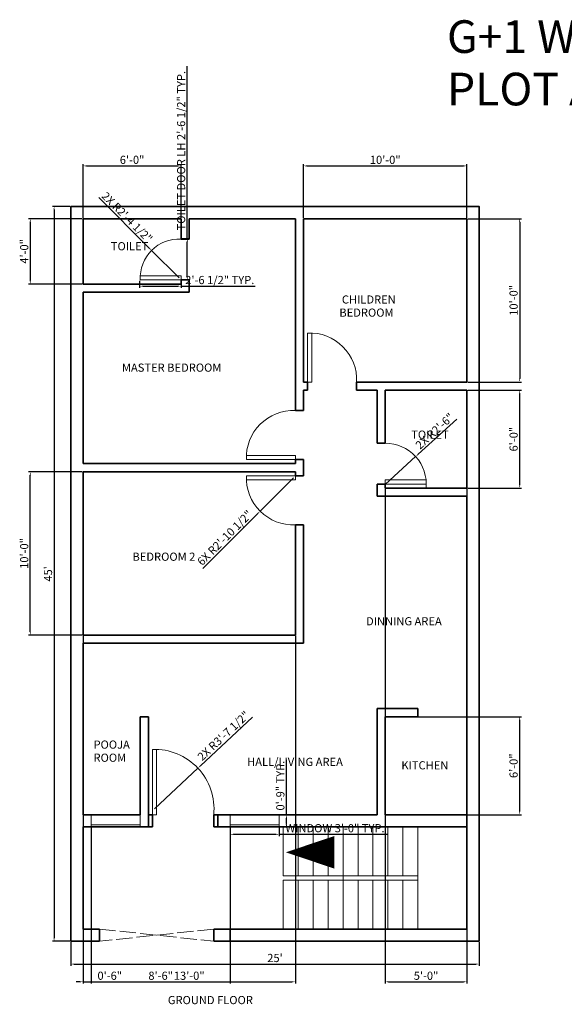
# Model space of a CAD drawing. Units: inches. Extents: x 740 to 2438, y 2555 to 3278.
# Tile 2 of 3: x 1188 to 1588, y 2555 to 3278. Entities that reach past the tile are written whole.
import ezdxf

# ---------------------------------------------------------------- set-up
doc = ezdxf.new("R2010")
doc.units = ezdxf.units.IN
doc.linetypes.add('ACAD_ISO02W100', pattern=[15, 12, -3])
for name, color, linetype, lineweight in [('A-ANNO-DIMS', 2, 'Continuous', 18), ('A-ANNO-TEXT', 7, 'Continuous', 18), ('A-AREA-IDEN', 7, 'Continuous', 18), ('A-DOOR', 3, 'Continuous', 18), ('A-DOOR-SWNG', 3, 'ACAD_ISO02W100', 13), ('A-FLOR-STRS', 7, 'Continuous', 18), ('A-FLOR-STRS-PATH', 2, 'ACAD_ISO02W100', 13), ('A-GLAZ', 4, 'Continuous', 18), ('A-WALL', 7, 'Continuous', 35)]:
    doc.layers.add(name, color=color, linetype=linetype, lineweight=lineweight)
doc.styles.get("Standard").update_dxf_attribs({"font": 'arial.ttf'})
doc.dimstyles.new('ISO-25', dxfattribs={"dimtxt": 6, "dimasz": 2.5, "dimexe": 1.25, "dimexo": 0.625, "dimtad": 1, "dimdec": 1, "dimlunit": 3, "dimtxsty": 'Standard', "dimcen": 2.5, "dimadec": 0, "dimazin": 0, "dimtfac": 1, "dimtdec": 1, "dimtmove": 0, "dimatfit": 3, "dimfxl": 1, "dimarcsym": 0})

# ---------------------------------------------------------------- blocks, each defined once
blk = doc.blocks.new('*D1')
at = {"layer": 'A-ANNO-DIMS', "color": 0, "lineweight": -2, "transparency": 16777216}
for p, q in [((1225.87, 2600.59), (1225.87, 2583.21)), ((1525.87, 2600.59), (1525.87, 2583.21)), ((1228.37, 2584.46), (1523.37, 2584.46))]:
    blk.add_line(p, q, dxfattribs=at)
at = {"layer": 'A-ANNO-DIMS', "color": 0, "transparency": 16777216}
for points in [[(1228.37, 2584.87), (1228.37, 2584.04), (1225.87, 2584.46)], [(1523.37, 2584.87), (1523.37, 2584.04), (1525.87, 2584.46)]]:
    blk.add_solid(points, dxfattribs=at)
at = {"layer": 'Defpoints', "color": 0, "transparency": 16777216}
for p in [(1225.87, 2601.21), (1525.87, 2601.21), (1525.87, 2584.46)]:
    blk.add_point(p, dxfattribs=at)
at = {"layer": 'A-ANNO-DIMS', "color": 0, "transparency": 16777216, "insert": (1375.87, 2588.15), "char_height": 6, "attachment_point": 5}
blk.add_mtext("25'", dxfattribs=at)
blk = doc.blocks.new('*D2')
at = {"layer": 'A-ANNO-DIMS', "color": 0, "lineweight": -2, "transparency": 16777216}
for p, q in [((1225.24, 3141.21), (1212.31, 3141.21)), ((1213.56, 3138.71), (1213.56, 2603.71)), ((1225.24, 2601.21), (1212.31, 2601.21))]:
    blk.add_line(p, q, dxfattribs=at)
at = {"layer": 'A-ANNO-DIMS', "color": 0, "transparency": 16777216}
for points in [[(1213.15, 3138.71), (1213.98, 3138.71), (1213.56, 3141.21)], [(1213.15, 2603.71), (1213.98, 2603.71), (1213.56, 2601.21)]]:
    blk.add_solid(points, dxfattribs=at)
at = {"layer": 'Defpoints', "color": 0, "transparency": 16777216}
for p in [(1225.87, 3141.21), (1213.56, 2601.21), (1225.87, 2601.21)]:
    blk.add_point(p, dxfattribs=at)
at = {"layer": 'A-ANNO-DIMS', "color": 0, "transparency": 16777216, "insert": (1209.89, 2871.21), "char_height": 6, "attachment_point": 5, "rotation": 90}
blk.add_mtext("45'", dxfattribs=at)
blk = doc.blocks.new('DOOR-PLAN-48')
blk.add_lwpolyline([(0, 0), (3, 0), (3, 48), (0, 48)], close=True)
blk.add_arc((1.5, 4.3125), 43.7132, 354.3383149, 91.9664646)
blk = doc.blocks.new('DOOR-PLAN-36')
blk.add_lwpolyline([(36, 36), (0, 36), (0, 33), (36, 33)], close=True)
blk.add_arc((34.5, 34.5), 34.53, 177.51045, 272.48955)
blk = doc.blocks.new('DOOR-PLAN-30-L')
blk.add_lwpolyline([(30, 0), (0, 0), (0, 3), (30, 3)], close=True)
blk.add_arc((28.5, 1.5), 28.54, 86.98721, 183.01279)
blk = doc.blocks.new('DOOR-PLAN-30-R')
blk.add_lwpolyline([(0, 3), (30, 3), (30, 6), (0, 6)], close=True)
blk.add_arc((0.15, 3), 30, 354.2609, 90.28648)
blk = doc.blocks.new('STAIR-PLAN-RETURN')
for p, q in [((0, 75), (0, 39)), ((11, 75), (11, 39)), ((22, 75), (22, 39)), ((33, 75), (33, 39)), ((44, 75), (44, 0)), ((55, 75), (55, 39)), ((66, 75), (66, 39)), ((77, 75), (77, 39)), ((88, 75), (88, 39)), ((99, 75), (99, 0)), ((0, 39), (99, 39)), ((0, 36), (99, 36)), ((0, 36), (0, 0)), ((11, 36), (11, 0)), ((22, 36), (22, 0)), ((33, 36), (33, 0)), ((55, 36), (55, 0)), ((66, 36), (66, 0)), ((77, 36), (77, 0)), ((88, 36), (88, 0))]:
    blk.add_line(p, q)
blk = doc.blocks.new('STAIR-PATH-RETURN')
for points in [[(15.6, 0, 0, 0, 0), (114.75, 0, 0, 0, 0), (114.75, 41.58, 0, 0, 0), (35.71, 41.58, 96, 0, 0)], [(35.71, 41.58, 24, 0, 0), (0, 41.58, 0, 0, 0)]]:
    blk.add_lwpolyline(points, format="xyseb")
blk = doc.blocks.new('WINDOW-PLAN-36')
blk.add_line((0, 1.5), (36, 1.5))
blk.add_lwpolyline([(0, 0), (0, 9), (36, 9), (36, 0)], close=True)
blk = doc.blocks.new('*D28')
at = {"layer": 'A-ANNO-DIMS', "color": 0, "lineweight": -2, "transparency": 16777216}
for p, q in [((1311.43, 3117.64), (1311.43, 3244.28)), ((1307.49, 3117.64), (1312.68, 3117.64)), ((1311.43, 3089.71), (1311.43, 3115.14)), ((1307.49, 3087.21), (1312.68, 3087.21))]:
    blk.add_line(p, q, dxfattribs=at)
at = {"layer": 'A-ANNO-DIMS', "color": 0, "transparency": 16777216}
for points in [[(1311.01, 3115.14), (1311.85, 3115.14), (1311.43, 3117.64)], [(1311.01, 3089.71), (1311.85, 3089.71), (1311.43, 3087.21)]]:
    blk.add_solid(points, dxfattribs=at)
at = {"layer": 'Defpoints', "color": 0, "transparency": 16777216}
for p in [(1306.87, 3117.64), (1311.43, 3117.64), (1306.87, 3087.21)]:
    blk.add_point(p, dxfattribs=at)
at = {"layer": 'A-ANNO-DIMS', "color": 0, "transparency": 16777216, "insert": (1307.7, 3182.21), "char_height": 6, "attachment_point": 5, "rotation": 90}
blk.add_mtext('TOILET DOOR LH 2\'-6 1/2" TYP.', dxfattribs=at)
blk = doc.blocks.new('*D29')
at = {"layer": 'A-ANNO-DIMS', "color": 0, "lineweight": -2, "transparency": 16777216}
for p, q in [((1276.44, 3086.59), (1276.44, 3081.4)), ((1278.94, 3082.65), (1304.37, 3082.65)), ((1306.87, 3086.59), (1306.87, 3081.4)), ((1306.87, 3082.65), (1361.27, 3082.65))]:
    blk.add_line(p, q, dxfattribs=at)
at = {"layer": 'A-ANNO-DIMS', "color": 0, "transparency": 16777216}
for points in [[(1278.94, 3083.07), (1278.94, 3082.23), (1276.44, 3082.65)], [(1304.37, 3083.07), (1304.37, 3082.23), (1306.87, 3082.65)]]:
    blk.add_solid(points, dxfattribs=at)
at = {"layer": 'Defpoints', "color": 0, "transparency": 16777216}
for p in [(1276.44, 3087.21), (1306.87, 3087.21), (1306.87, 3082.65)]:
    blk.add_point(p, dxfattribs=at)
at = {"layer": 'A-ANNO-DIMS', "color": 0, "transparency": 16777216, "insert": (1335.32, 3086.38), "char_height": 6, "attachment_point": 5}
blk.add_mtext('2\'-6 1/2" TYP.', dxfattribs=at)
blk = doc.blocks.new('*D32')
at = {"layer": 'A-ANNO-DIMS', "color": 0, "lineweight": -2, "transparency": 16777216}
for p, q in [((1342.87, 2684.59), (1342.87, 2678.56)), ((1378.87, 2684.59), (1378.87, 2678.56)), ((1345.37, 2679.81), (1376.37, 2679.81)), ((1378.87, 2679.81), (1458.54, 2679.81))]:
    blk.add_line(p, q, dxfattribs=at)
at = {"layer": 'A-ANNO-DIMS', "color": 0, "transparency": 16777216}
for points in [[(1345.37, 2680.23), (1345.37, 2679.4), (1342.87, 2679.81)], [(1376.37, 2680.23), (1376.37, 2679.4), (1378.87, 2679.81)]]:
    blk.add_solid(points, dxfattribs=at)
at = {"layer": 'Defpoints', "color": 0, "transparency": 16777216}
for p in [(1342.87, 2685.21), (1378.87, 2685.21), (1378.87, 2679.81)]:
    blk.add_point(p, dxfattribs=at)
at = {"layer": 'A-ANNO-DIMS', "color": 0, "transparency": 16777216, "insert": (1419.95, 2683.54), "char_height": 6, "attachment_point": 5}
blk.add_mtext('WINDOW 3\'-0" TYP.', dxfattribs=at)
blk = doc.blocks.new('*D33')
at = {"layer": 'A-ANNO-DIMS', "color": 0, "lineweight": -2, "transparency": 16777216}
for p, q in [((1384.27, 2694.21), (1384.27, 2734.54)), ((1379.49, 2694.21), (1385.52, 2694.21)), ((1379.49, 2685.21), (1385.52, 2685.21)), ((1384.27, 2687.71), (1384.27, 2691.71))]:
    blk.add_line(p, q, dxfattribs=at)
at = {"layer": 'A-ANNO-DIMS', "color": 0, "transparency": 16777216}
for points in [[(1383.85, 2691.71), (1384.68, 2691.71), (1384.27, 2694.21)], [(1383.85, 2687.71), (1384.68, 2687.71), (1384.27, 2685.21)]]:
    blk.add_solid(points, dxfattribs=at)
at = {"layer": 'Defpoints', "color": 0, "transparency": 16777216}
for p in [(1378.87, 2694.21), (1384.27, 2694.21), (1378.87, 2685.21)]:
    blk.add_point(p, dxfattribs=at)
at = {"layer": 'A-ANNO-DIMS', "color": 0, "transparency": 16777216, "insert": (1380.58, 2715.62), "char_height": 6, "attachment_point": 5, "rotation": 90}
blk.add_mtext('0\'-9" TYP.', dxfattribs=at)
blk = doc.blocks.new('*D61')
at = {"layer": 'A-ANNO-DIMS', "color": 0, "lineweight": -2, "transparency": 16777216}
for p, q in [((1234.87, 2825.59), (1234.87, 2570.16)), ((1390.87, 2825.59), (1390.87, 2570.16)), ((1237.37, 2571.41), (1388.37, 2571.41))]:
    blk.add_line(p, q, dxfattribs=at)
at = {"layer": 'A-ANNO-DIMS', "color": 0, "transparency": 16777216}
for points in [[(1237.37, 2571.83), (1237.37, 2571), (1234.87, 2571.41)], [(1388.37, 2571.83), (1388.37, 2571), (1390.87, 2571.41)]]:
    blk.add_solid(points, dxfattribs=at)
at = {"layer": 'Defpoints', "color": 0, "transparency": 16777216}
for p in [(1234.87, 2826.21), (1390.87, 2826.21), (1390.87, 2571.41)]:
    blk.add_point(p, dxfattribs=at)
at = {"layer": 'A-ANNO-DIMS', "color": 0, "transparency": 16777216, "insert": (1312.87, 2575.1), "char_height": 6, "attachment_point": 5}
blk.add_mtext('13\'-0"', dxfattribs=at)
blk = doc.blocks.new('*D62')
at = {"layer": 'A-ANNO-DIMS', "color": 0, "lineweight": -2, "transparency": 16777216}
for p, q in [((1234.24, 2946.21), (1194.82, 2946.21)), ((1196.07, 2828.71), (1196.07, 2943.71)), ((1234.24, 2826.21), (1194.82, 2826.21))]:
    blk.add_line(p, q, dxfattribs=at)
at = {"layer": 'A-ANNO-DIMS', "color": 0, "transparency": 16777216}
for points in [[(1195.65, 2943.71), (1196.48, 2943.71), (1196.07, 2946.21)], [(1195.65, 2828.71), (1196.48, 2828.71), (1196.07, 2826.21)]]:
    blk.add_solid(points, dxfattribs=at)
at = {"layer": 'Defpoints', "color": 0, "transparency": 16777216}
for p in [(1196.07, 2946.21), (1234.87, 2946.21), (1234.87, 2826.21)]:
    blk.add_point(p, dxfattribs=at)
at = {"layer": 'A-ANNO-DIMS', "color": 0, "transparency": 16777216, "insert": (1192.38, 2886.21), "char_height": 6, "attachment_point": 5, "rotation": 90}
blk.add_mtext('10\'-0"', dxfattribs=at)
blk = doc.blocks.new('*D63')
at = {"layer": 'A-ANNO-DIMS', "color": 0, "lineweight": -2, "transparency": 16777216}
for p, q in [((1396.87, 3132.84), (1396.87, 3172.26)), ((1399.37, 3171.01), (1514.37, 3171.01)), ((1516.87, 3132.84), (1516.87, 3172.26))]:
    blk.add_line(p, q, dxfattribs=at)
at = {"layer": 'A-ANNO-DIMS', "color": 0, "transparency": 16777216}
for points in [[(1399.37, 3171.43), (1399.37, 3170.6), (1396.87, 3171.01)], [(1514.37, 3171.43), (1514.37, 3170.6), (1516.87, 3171.01)]]:
    blk.add_solid(points, dxfattribs=at)
at = {"layer": 'Defpoints', "color": 0, "transparency": 16777216}
for p in [(1516.87, 3171.01), (1396.87, 3132.21), (1516.87, 3132.21)]:
    blk.add_point(p, dxfattribs=at)
at = {"layer": 'A-ANNO-DIMS', "color": 0, "transparency": 16777216, "insert": (1456.87, 3174.7), "char_height": 6, "attachment_point": 5}
blk.add_mtext('10\'-0"', dxfattribs=at)
blk = doc.blocks.new('*D64')
at = {"layer": 'A-ANNO-DIMS', "color": 0, "lineweight": -2, "transparency": 16777216}
for p, q in [((1517.49, 3132.21), (1556.92, 3132.21)), ((1555.67, 3129.71), (1555.67, 3014.71)), ((1517.49, 3012.21), (1556.92, 3012.21))]:
    blk.add_line(p, q, dxfattribs=at)
at = {"layer": 'A-ANNO-DIMS', "color": 0, "transparency": 16777216}
for points in [[(1555.25, 3129.71), (1556.08, 3129.71), (1555.67, 3132.21)], [(1555.25, 3014.71), (1556.08, 3014.71), (1555.67, 3012.21)]]:
    blk.add_solid(points, dxfattribs=at)
at = {"layer": 'Defpoints', "color": 0, "transparency": 16777216}
for p in [(1516.87, 3132.21), (1516.87, 3012.21), (1555.67, 3012.21)]:
    blk.add_point(p, dxfattribs=at)
at = {"layer": 'A-ANNO-DIMS', "color": 0, "transparency": 16777216, "insert": (1551.98, 3072.21), "char_height": 6, "attachment_point": 5, "rotation": 90}
blk.add_mtext('10\'-0"', dxfattribs=at)
blk = doc.blocks.new('*D65')
at = {"layer": 'A-ANNO-DIMS', "color": 0, "lineweight": -2, "transparency": 16777216}
for p, q in [((1234.87, 3132.84), (1234.87, 3172.26)), ((1237.37, 3171.01), (1304.37, 3171.01)), ((1306.87, 3132.84), (1306.87, 3172.26))]:
    blk.add_line(p, q, dxfattribs=at)
at = {"layer": 'A-ANNO-DIMS', "color": 0, "transparency": 16777216}
for points in [[(1237.37, 3171.43), (1237.37, 3170.6), (1234.87, 3171.01)], [(1304.37, 3171.43), (1304.37, 3170.6), (1306.87, 3171.01)]]:
    blk.add_solid(points, dxfattribs=at)
at = {"layer": 'Defpoints', "color": 0, "transparency": 16777216}
for p in [(1306.87, 3171.01), (1234.87, 3132.21), (1306.87, 3132.21)]:
    blk.add_point(p, dxfattribs=at)
at = {"layer": 'A-ANNO-DIMS', "color": 0, "transparency": 16777216, "insert": (1270.87, 3174.7), "char_height": 6, "attachment_point": 5}
blk.add_mtext('6\'-0"', dxfattribs=at)
blk = doc.blocks.new('*D66')
at = {"layer": 'A-ANNO-DIMS', "color": 0, "lineweight": -2, "transparency": 16777216}
for p, q in [((1234.24, 3132.21), (1194.82, 3132.21)), ((1196.07, 3129.71), (1196.07, 3086.71)), ((1234.24, 3084.21), (1194.82, 3084.21))]:
    blk.add_line(p, q, dxfattribs=at)
at = {"layer": 'A-ANNO-DIMS', "color": 0, "transparency": 16777216}
for points in [[(1195.65, 3129.71), (1196.48, 3129.71), (1196.07, 3132.21)], [(1195.65, 3086.71), (1196.48, 3086.71), (1196.07, 3084.21)]]:
    blk.add_solid(points, dxfattribs=at)
at = {"layer": 'Defpoints', "color": 0, "transparency": 16777216}
for p in [(1234.87, 3132.21), (1196.07, 3084.21), (1234.87, 3084.21)]:
    blk.add_point(p, dxfattribs=at)
at = {"layer": 'A-ANNO-DIMS', "color": 0, "transparency": 16777216, "insert": (1192.38, 3108.21), "char_height": 6, "attachment_point": 5, "rotation": 90}
blk.add_mtext('4\'-0"', dxfattribs=at)
blk = doc.blocks.new('*D67')
at = {"layer": 'A-ANNO-DIMS', "color": 0, "lineweight": -2, "transparency": 16777216}
for p, q in [((1456.87, 2933.59), (1456.87, 2570.16)), ((1516.87, 2933.59), (1516.87, 2570.16)), ((1459.37, 2571.41), (1514.37, 2571.41))]:
    blk.add_line(p, q, dxfattribs=at)
at = {"layer": 'A-ANNO-DIMS', "color": 0, "transparency": 16777216}
for points in [[(1459.37, 2571.83), (1459.37, 2571), (1456.87, 2571.41)], [(1514.37, 2571.83), (1514.37, 2571), (1516.87, 2571.41)]]:
    blk.add_solid(points, dxfattribs=at)
at = {"layer": 'Defpoints', "color": 0, "transparency": 16777216}
for p in [(1456.87, 2934.21), (1516.87, 2934.21), (1516.87, 2571.41)]:
    blk.add_point(p, dxfattribs=at)
at = {"layer": 'A-ANNO-DIMS', "color": 0, "transparency": 16777216, "insert": (1486.87, 2575.1), "char_height": 6, "attachment_point": 5}
blk.add_mtext('5\'-0"', dxfattribs=at)
blk = doc.blocks.new('*D68')
at = {"layer": 'A-ANNO-DIMS', "color": 0, "lineweight": -2, "transparency": 16777216}
for p, q in [((1517.49, 3006.21), (1556.92, 3006.21)), ((1555.67, 2936.71), (1555.67, 3003.71)), ((1517.49, 2934.21), (1556.92, 2934.21))]:
    blk.add_line(p, q, dxfattribs=at)
at = {"layer": 'A-ANNO-DIMS', "color": 0, "transparency": 16777216}
for points in [[(1555.25, 3003.71), (1556.08, 3003.71), (1555.67, 3006.21)], [(1555.25, 2936.71), (1556.08, 2936.71), (1555.67, 2934.21)]]:
    blk.add_solid(points, dxfattribs=at)
at = {"layer": 'Defpoints', "color": 0, "transparency": 16777216}
for p in [(1516.87, 3006.21), (1555.67, 3006.21), (1516.87, 2934.21)]:
    blk.add_point(p, dxfattribs=at)
at = {"layer": 'A-ANNO-DIMS', "color": 0, "transparency": 16777216, "insert": (1551.98, 2970.21), "char_height": 6, "attachment_point": 5, "rotation": 90}
blk.add_mtext('6\'-0"', dxfattribs=at)
blk = doc.blocks.new('*D69')
at = {"layer": 'A-ANNO-DIMS', "color": 0, "lineweight": -2, "transparency": 16777216}
for p, q in [((1456.87, 2693.59), (1456.87, 2570.16)), ((1516.87, 2693.59), (1516.87, 2570.16)), ((1459.37, 2571.41), (1514.37, 2571.41))]:
    blk.add_line(p, q, dxfattribs=at)
at = {"layer": 'A-ANNO-DIMS', "color": 0, "transparency": 16777216}
for points in [[(1459.37, 2571.83), (1459.37, 2571), (1456.87, 2571.41)], [(1514.37, 2571.83), (1514.37, 2571), (1516.87, 2571.41)]]:
    blk.add_solid(points, dxfattribs=at)
at = {"layer": 'Defpoints', "color": 0, "transparency": 16777216}
for p in [(1456.87, 2694.21), (1516.87, 2694.21), (1516.87, 2571.41)]:
    blk.add_point(p, dxfattribs=at)
at = {"layer": 'A-ANNO-DIMS', "color": 0, "transparency": 16777216, "insert": (1486.87, 2575.1), "char_height": 6, "attachment_point": 5}
blk.add_mtext('5\'-0"', dxfattribs=at)
blk = doc.blocks.new('*D70')
at = {"layer": 'A-ANNO-DIMS', "color": 0, "lineweight": -2, "transparency": 16777216}
for p, q in [((1457.49, 2766.21), (1556.92, 2766.21)), ((1555.67, 2696.71), (1555.67, 2763.71)), ((1457.49, 2694.21), (1556.92, 2694.21))]:
    blk.add_line(p, q, dxfattribs=at)
at = {"layer": 'A-ANNO-DIMS', "color": 0, "transparency": 16777216}
for points in [[(1555.25, 2763.71), (1556.08, 2763.71), (1555.67, 2766.21)], [(1555.25, 2696.71), (1556.08, 2696.71), (1555.67, 2694.21)]]:
    blk.add_solid(points, dxfattribs=at)
at = {"layer": 'Defpoints', "color": 0, "transparency": 16777216}
for p in [(1456.87, 2766.21), (1555.67, 2766.21), (1456.87, 2694.21)]:
    blk.add_point(p, dxfattribs=at)
at = {"layer": 'A-ANNO-DIMS', "color": 0, "transparency": 16777216, "insert": (1551.98, 2730.21), "char_height": 6, "attachment_point": 5, "rotation": 90}
blk.add_mtext('6\'-0"', dxfattribs=at)
blk = doc.blocks.new('*D76')
at = {"layer": 'A-ANNO-DIMS', "color": 0, "lineweight": -2, "transparency": 16777216}
for p, q in [((1234.87, 2693.59), (1234.87, 2570.16)), ((1240.87, 2684.59), (1240.87, 2570.16)), ((1232.37, 2571.41), (1229.87, 2571.41)), ((1234.87, 2571.41), (1240.87, 2571.41)), ((1243.37, 2571.41), (1263.07, 2571.41))]:
    blk.add_line(p, q, dxfattribs=at)
at = {"layer": 'A-ANNO-DIMS', "color": 0, "transparency": 16777216}
for points in [[(1232.37, 2571.83), (1232.37, 2571), (1234.87, 2571.41)], [(1243.37, 2571.83), (1243.37, 2571), (1240.87, 2571.41)]]:
    blk.add_solid(points, dxfattribs=at)
at = {"layer": 'Defpoints', "color": 0, "transparency": 16777216}
for p in [(1234.87, 2694.21), (1240.87, 2685.21), (1240.87, 2571.41)]:
    blk.add_point(p, dxfattribs=at)
at = {"layer": 'A-ANNO-DIMS', "color": 0, "transparency": 16777216, "insert": (1254.47, 2575.1), "char_height": 6, "attachment_point": 5}
blk.add_mtext('0\'-6"', dxfattribs=at)
blk = doc.blocks.new('*D77')
at = {"layer": 'A-ANNO-DIMS', "color": 0, "lineweight": -2, "transparency": 16777216}
for p, q in [((1240.87, 2684.59), (1240.87, 2570.16)), ((1342.87, 2684.59), (1342.87, 2570.16)), ((1243.37, 2571.41), (1340.37, 2571.41))]:
    blk.add_line(p, q, dxfattribs=at)
at = {"layer": 'A-ANNO-DIMS', "color": 0, "transparency": 16777216}
for points in [[(1243.37, 2571.83), (1243.37, 2571), (1240.87, 2571.41)], [(1340.37, 2571.83), (1340.37, 2571), (1342.87, 2571.41)]]:
    blk.add_solid(points, dxfattribs=at)
at = {"layer": 'Defpoints', "color": 0, "transparency": 16777216}
for p in [(1240.87, 2685.21), (1342.87, 2685.21), (1342.87, 2571.41)]:
    blk.add_point(p, dxfattribs=at)
at = {"layer": 'A-ANNO-DIMS', "color": 0, "transparency": 16777216, "insert": (1291.87, 2575.1), "char_height": 6, "attachment_point": 5}
blk.add_mtext('8\'-6"', dxfattribs=at)
blk = doc.blocks.new('*D79')
at = {"layer": 'A-ANNO-DIMS', "color": 0, "lineweight": -2, "transparency": 16777216}
for p, q in [((1359.32, 2765.98), (1321.08, 2730.13)), ((1287.37, 2698.53), (1319.26, 2728.42))]:
    blk.add_line(p, q, dxfattribs=at)
at = {"layer": 'A-ANNO-DIMS', "color": 0, "transparency": 16777216}
blk.add_solid([(1320.8, 2730.44), (1321.37, 2729.83), (1319.26, 2728.42)], dxfattribs=at)
at = {"layer": 'Defpoints', "color": 0, "transparency": 16777216}
for p in [(1319.26, 2728.42), (1287.37, 2698.53)]:
    blk.add_point(p, dxfattribs=at)
at = {"layer": 'A-ANNO-DIMS', "color": 0, "transparency": 16777216, "insert": (1338.56, 2751.63), "char_height": 6, "attachment_point": 5, "rotation": 43.15246}
blk.add_mtext('2X R3\'-7 1/2"', dxfattribs=at)
blk = doc.blocks.new('*D80')
at = {"layer": 'A-ANNO-DIMS', "color": 0, "lineweight": -2, "transparency": 16777216}
for p, q in [((1389.37, 2941.71), (1364.95, 2917.29)), ((1322.87, 2875.22), (1363.18, 2915.53))]:
    blk.add_line(p, q, dxfattribs=at)
at = {"layer": 'A-ANNO-DIMS', "color": 0, "transparency": 16777216}
blk.add_solid([(1362.89, 2915.82), (1363.47, 2915.23), (1364.95, 2917.29)], dxfattribs=at)
at = {"layer": 'Defpoints', "color": 0, "transparency": 16777216}
for p in [(1389.37, 2941.71), (1364.95, 2917.29)]:
    blk.add_point(p, dxfattribs=at)
at = {"layer": 'A-ANNO-DIMS', "color": 0, "transparency": 16777216, "insert": (1339.5, 2897.12), "char_height": 6, "attachment_point": 5, "rotation": 44.99952}
blk.add_mtext('6X R2\'-10 1/2"', dxfattribs=at)
blk = doc.blocks.new('*D81')
at = {"layer": 'A-ANNO-DIMS', "color": 0, "lineweight": -2, "transparency": 16777216}
for p, q in [((1509.51, 2984.93), (1481.06, 2959.07)), ((1457.02, 2937.21), (1479.22, 2957.39))]:
    blk.add_line(p, q, dxfattribs=at)
at = {"layer": 'A-ANNO-DIMS', "color": 0, "transparency": 16777216}
blk.add_solid([(1480.78, 2959.38), (1481.35, 2958.77), (1479.22, 2957.39)], dxfattribs=at)
at = {"layer": 'Defpoints', "color": 0, "transparency": 16777216}
for p in [(1479.22, 2957.39), (1457.02, 2937.21)]:
    blk.add_point(p, dxfattribs=at)
at = {"layer": 'A-ANNO-DIMS', "color": 0, "transparency": 16777216, "insert": (1493.73, 2975.57), "char_height": 6, "attachment_point": 5, "rotation": 42.27293}
blk.add_mtext('2X R2\'-6"', dxfattribs=at)
blk = doc.blocks.new('*D82')
at = {"layer": 'A-ANNO-DIMS', "color": 0, "lineweight": -2, "transparency": 16777216}
for p, q in [((1246.35, 3147.73), (1283.42, 3110.66)), ((1305.37, 3088.71), (1285.19, 3108.89))]:
    blk.add_line(p, q, dxfattribs=at)
at = {"layer": 'A-ANNO-DIMS', "color": 0, "transparency": 16777216}
blk.add_solid([(1283.71, 3110.96), (1283.12, 3110.37), (1285.19, 3108.89)], dxfattribs=at)
at = {"layer": 'Defpoints', "color": 0, "transparency": 16777216}
for p in [(1285.19, 3108.89), (1305.37, 3088.71)]:
    blk.add_point(p, dxfattribs=at)
at = {"layer": 'A-ANNO-DIMS', "color": 0, "transparency": 16777216, "insert": (1266.64, 3132.71), "char_height": 6, "attachment_point": 5, "rotation": 315.00046}
blk.add_mtext('2X R2\'-4 1/2"', dxfattribs=at)

msp = doc.modelspace()

# ---------------------------------------------------------------- linework, layer by layer
at = {"layer": 'A-DOOR-SWNG'}
for p, q in [((1246.87, 2610.21), (1330.87, 2601.21)), ((1330.87, 2610.21), (1246.87, 2601.21))]:
    msp.add_line(p, q, dxfattribs=at)
at = {"layer": 'A-WALL'}
for p, q in [((1234.87, 3132.21), (1306.87, 3132.21)), ((1234.87, 3084.21), (1234.87, 3132.21)), ((1306.87, 3117.21), (1306.87, 3132.21)), ((1312.87, 3132.21), (1390.87, 3132.21)), ((1312.87, 3117.21), (1312.87, 3132.21)), ((1390.87, 3132.21), (1390.87, 2991.21)), ((1396.87, 3132.21), (1396.87, 3012.21)), ((1396.87, 3132.21), (1516.87, 3132.21)), ((1516.87, 3132.21), (1516.87, 3012.21)), ((1306.87, 3117.21), (1312.87, 3117.21)), ((1234.87, 3084.21), (1306.87, 3084.21)), ((1306.87, 3084.21), (1306.87, 3087.21)), ((1306.87, 3084.21), (1306.87, 3087.21)), ((1306.87, 3087.21), (1312.87, 3087.21)), ((1312.87, 3078.21), (1312.87, 3087.21)), ((1234.87, 2952.21), (1234.87, 3078.21)), ((1234.87, 3078.21), (1312.87, 3078.21)), ((1396.87, 3012.21), (1399.87, 3012.21)), ((1396.87, 3012.21), (1399.87, 3012.21)), ((1399.87, 3012.21), (1399.87, 3006.21)), ((1435.87, 3012.21), (1435.87, 3006.21)), ((1435.87, 3012.21), (1516.87, 3012.21)), ((1396.87, 3006.21), (1399.87, 3006.21)), ((1396.87, 3006.21), (1396.87, 2991.21)), ((1435.87, 3006.21), (1450.87, 3006.21)), ((1450.87, 3006.21), (1450.87, 2967.21)), ((1456.87, 3006.21), (1456.87, 2967.21)), ((1456.87, 3006.21), (1516.87, 3006.21)), ((1516.87, 3006.21), (1516.87, 2934.21)), ((1390.87, 2991.21), (1396.87, 2991.21)), ((1456.87, 2967.21), (1450.87, 2967.21)), ((1390.87, 2952.21), (1390.87, 2955.21)), ((1390.87, 2955.21), (1396.87, 2955.21)), ((1390.87, 2955.21), (1390.87, 2952.21)), ((1396.87, 2955.21), (1396.87, 2943.21)), ((1234.87, 2952.21), (1390.87, 2952.21)), ((1234.87, 2946.21), (1390.87, 2946.21)), ((1234.87, 2826.21), (1234.87, 2946.21)), ((1390.87, 2946.21), (1390.87, 2943.21)), ((1390.87, 2946.21), (1390.87, 2943.21)), ((1390.87, 2943.21), (1396.87, 2943.21)), ((1456.87, 2937.21), (1450.87, 2937.21)), ((1450.87, 2937.21), (1450.87, 2928.21)), ((1456.87, 2934.21), (1456.87, 2937.21)), ((1456.87, 2937.21), (1456.87, 2934.21)), ((1456.87, 2934.21), (1516.87, 2934.21)), ((1450.87, 2928.21), (1516.87, 2928.21)), ((1516.87, 2928.21), (1516.87, 2610.21)), ((1390.87, 2907.21), (1396.87, 2907.21)), ((1390.87, 2907.21), (1390.87, 2826.21)), ((1396.87, 2907.21), (1396.87, 2820.21)), ((1234.87, 2826.21), (1390.87, 2826.21)), ((1234.87, 2820.21), (1396.87, 2820.21)), ((1234.87, 2694.21), (1234.87, 2820.21)), ((1480.87, 2772.21), (1450.87, 2772.21)), ((1450.87, 2772.21), (1450.87, 2766.21)), ((1480.87, 2766.21), (1480.87, 2772.21)), ((1282.87, 2766.21), (1276.87, 2766.21)), ((1276.87, 2766.21), (1276.87, 2694.21)), ((1282.87, 2694.21), (1282.87, 2766.21)), ((1450.87, 2766.21), (1450.87, 2694.21)), ((1456.87, 2694.21), (1456.87, 2766.21)), ((1456.87, 2766.21), (1480.87, 2766.21)), ((1276.87, 2694.21), (1234.87, 2694.21)), ((1282.87, 2694.21), (1282.87, 2685.21)), ((1282.87, 2694.21), (1285.87, 2694.21)), ((1285.87, 2694.21), (1285.87, 2685.21)), ((1330.87, 2694.21), (1330.87, 2685.21)), ((1450.87, 2694.21), (1330.87, 2694.21)), ((1333.87, 2694.21), (1333.87, 2685.21)), ((1516.87, 2694.21), (1456.87, 2694.21)), ((1234.87, 2610.21), (1234.87, 2685.21)), ((1282.87, 2685.21), (1234.87, 2685.21)), ((1285.87, 2685.21), (1282.87, 2685.21)), ((1516.87, 2685.21), (1330.87, 2685.21)), ((1234.87, 2610.21), (1246.87, 2610.21)), ((1246.87, 2610.21), (1234.87, 2610.21)), ((1246.87, 2610.21), (1246.87, 2601.21)), ((1516.87, 2610.21), (1330.87, 2610.21)), ((1330.87, 2610.21), (1330.87, 2601.21)), ((1342.87, 2610.21), (1342.87, 2601.21))]:
    msp.add_line(p, q, dxfattribs=at)
msp.add_lwpolyline([(1246.87, 2601.21), (1225.87, 2601.21), (1225.87, 3141.21), (1525.87, 3141.21), (1525.87, 2601.21), (1330.87, 2601.21)], dxfattribs=at)

# ---------------------------------------------------------------- block references
at = {"layer": 'A-DOOR'}
for name, p in [('DOOR-PLAN-30-L', (1276.87, 3087.21)), ('DOOR-PLAN-30-R', (1456.87, 2934.21)), ('DOOR-PLAN-36', (1354.87, 2907.21)), ('DOOR-PLAN-48', (1285.87, 2694.21))]:
    msp.add_blockref(name, p, dxfattribs=at)
at = {"layer": 'A-DOOR', "extrusion": (0, 0, -1), "zscale": -1}
for p, rotation in [((-1435.87, 3048.21), 269.9999999999956), ((-1354.87, 2991.21), 180)]:
    msp.add_blockref('DOOR-PLAN-36', p, dxfattribs=dict(at, rotation=rotation))
at = {"layer": 'A-FLOR-STRS'}
msp.add_blockref('STAIR-PLAN-RETURN', (1381.87, 2610.21), dxfattribs=at)
at = {"layer": 'A-FLOR-STRS-PATH'}
msp.add_blockref('STAIR-PATH-RETURN', (1383.86, 2625), dxfattribs=at)
at = {"layer": 'A-GLAZ'}
for p in [(1240.87, 2685.21), (1342.87, 2685.21)]:
    msp.add_blockref('WINDOW-PLAN-36', p, dxfattribs=at)

# ---------------------------------------------------------------- texts
at = {"layer": 'A-ANNO-TEXT'}
for s, height, p in [('G+1 WITH PENT HOUSE 3BHK', 24, (1502.24, 3254.05)), ("PLOT AREA:25'X45'", 24, (1502.24, 3215.5)), ('GROUND FLOOR', 6, (1297.14, 2554.99))]:
    msp.add_text(s, height=height, dxfattribs=at).set_placement(p)
at = {"layer": 'A-AREA-IDEN'}
for s, p in [('TOILET', (1255.24, 3109)), (' CHILDREN ', (1423.18, 3069.85)), ('BEDROOM', (1423.18, 3060.21)), ('MASTER BEDROOM', (1263.4, 3019.77)), ('TOILET', (1475.99, 2970.53)), ('BEDROOM 2', (1271.17, 2880.83)), ('DINNING AREA', (1442.78, 2833.39)), ('POOJA ', (1242.53, 2742.75)), ('ROOM', (1242.53, 2733.11)), ('HALL/LIVING AREA', (1355.41, 2730.03)), ('KITCHEN', (1468.74, 2727.52))]:
    msp.add_text(s, height=6, dxfattribs=at).set_placement(p)

# ---------------------------------------------------------------- dimensions: what is measured, and where the dimension line sits
at = {"layer": 'A-ANNO-DIMS'}
for base, p1, p2, text, picture, middle in [((1311.43, 3117.64), (1306.87, 3087.21), (1306.87, 3117.64), 'TOILET DOOR LH <> TYP.', '*D28', (1307.7, 3182.21)), ((1384.27, 2694.21), (1378.87, 2685.21), (1378.87, 2694.21), '<> TYP.', '*D33', (1380.58, 2715.62))]:
    dim = msp.add_linear_dim(base=base, p1=p1, p2=p2, angle=90, text=text, dimstyle='ISO-25', override={"dimdec": 1, "dimlfac": 1, "dimrnd": 0, "dimzin": 1, "dimdsep": 46, "dimlunit": 4, "dimfrac": 2}, dxfattribs=at)
    dim.commit()
    dim.dimension.update_dxf_attribs({"geometry": picture, "text_midpoint": middle})
for base, p1, p2, override, picture, middle in [((1306.87, 3171.01), (1234.87, 3132.21), (1306.87, 3132.21), {"dimdec": 1, "dimlfac": 1, "dimrnd": 0, "dimzin": 1, "dimdsep": 46, "dimlunit": 4, "dimfrac": 2}, '*D65', (1270.87, 3174.7)), ((1516.87, 3171.01), (1396.87, 3132.21), (1516.87, 3132.21), {"dimdec": 1, "dimlfac": 1, "dimrnd": 0, "dimzin": 1, "dimdsep": 46, "dimlunit": 4, "dimfrac": 2}, '*D63', (1456.87, 3174.7)), ((1516.87, 2571.41), (1456.87, 2934.21), (1516.87, 2934.21), {"dimdec": 1, "dimlfac": 1, "dimrnd": 0, "dimzin": 1, "dimdsep": 46, "dimlunit": 4, "dimfrac": 2}, '*D67', (1486.87, 2575.1)), ((1390.87, 2571.41), (1234.87, 2826.21), (1390.87, 2826.21), {"dimdec": 1, "dimlfac": 1, "dimrnd": 0, "dimzin": 1, "dimdsep": 46, "dimlunit": 4, "dimfrac": 2}, '*D61', (1312.87, 2575.1)), ((1240.87, 2571.41), (1234.87, 2694.21), (1240.87, 2685.21), {"dimdec": 1, "dimlfac": 1, "dimrnd": 0, "dimzin": 1, "dimdsep": 46, "dimlunit": 4, "dimfrac": 2}, '*D76', (1254.47, 2575.1)), ((1516.87, 2571.41), (1456.87, 2694.21), (1516.87, 2694.21), {"dimdec": 1, "dimlfac": 1, "dimrnd": 0, "dimzin": 1, "dimdsep": 46, "dimlunit": 4, "dimfrac": 2}, '*D69', (1486.87, 2575.1)), ((1342.87, 2571.41), (1240.87, 2685.21), (1342.87, 2685.21), {"dimdec": 1, "dimlfac": 1, "dimrnd": 0, "dimzin": 1, "dimdsep": 46, "dimlunit": 4, "dimfrac": 2}, '*D77', (1291.87, 2575.1)), ((1525.87, 2584.46), (1225.87, 2601.21), (1525.87, 2601.21), {"dimclrd": 0, "dimclre": 0, "dimclrt": 0}, '*D1', (1375.87, 2588.15))]:
    dim = msp.add_linear_dim(base=base, p1=p1, p2=p2, dimstyle='ISO-25', override=override, dxfattribs=at)
    dim.commit()
    dim.dimension.update_dxf_attribs({"geometry": picture, "text_midpoint": middle})
for center, mpoint, text, picture, middle in [((1305.37, 3088.71), (1285.19, 3108.89), '2X <>', '*D82', (1266.64, 3132.71)), ((1457.02, 2937.21), (1479.22, 2957.39), '2X <>', '*D81', (1493.73, 2975.57)), ((1389.37, 2941.71), (1364.95, 2917.29), '6X <>', '*D80', (1339.5, 2897.12)), ((1287.37, 2698.53), (1319.26, 2728.42), '2X <>', '*D79', (1338.56, 2751.63))]:
    dim = msp.add_radius_dim(center=center, mpoint=mpoint, text=text, dimstyle='ISO-25', override={"dimdec": 1, "dimlfac": 1, "dimrnd": 0, "dimzin": 1, "dimdsep": 46, "dimlunit": 4, "dimfrac": 2}, dxfattribs=at)
    dim.commit()
    dim.dimension.update_dxf_attribs({"geometry": picture, "text_midpoint": middle})
for base, p1, p2, override, picture, middle in [((1213.56, 2601.21), (1225.87, 3141.21), (1225.87, 2601.21), {"dimclrd": 0, "dimclre": 0, "dimclrt": 0}, '*D2', (1209.89, 2871.21)), ((1196.07, 3084.21), (1234.87, 3132.21), (1234.87, 3084.21), {"dimdec": 1, "dimlfac": 1, "dimrnd": 0, "dimzin": 1, "dimdsep": 46, "dimlunit": 4, "dimfrac": 2}, '*D66', (1192.38, 3108.21)), ((1555.67, 3012.21), (1516.87, 3132.21), (1516.87, 3012.21), {"dimdec": 1, "dimlfac": 1, "dimrnd": 0, "dimzin": 1, "dimdsep": 46, "dimlunit": 4, "dimfrac": 2}, '*D64', (1551.98, 3072.21)), ((1555.67, 3006.21), (1516.87, 2934.21), (1516.87, 3006.21), {"dimdec": 1, "dimlfac": 1, "dimrnd": 0, "dimzin": 1, "dimdsep": 46, "dimlunit": 4, "dimfrac": 2}, '*D68', (1551.98, 2970.21)), ((1196.07, 2946.21), (1234.87, 2826.21), (1234.87, 2946.21), {"dimdec": 1, "dimlfac": 1, "dimrnd": 0, "dimzin": 1, "dimdsep": 46, "dimlunit": 4, "dimfrac": 2}, '*D62', (1192.38, 2886.21)), ((1555.67, 2766.21), (1456.87, 2694.21), (1456.87, 2766.21), {"dimdec": 1, "dimlfac": 1, "dimrnd": 0, "dimzin": 1, "dimdsep": 46, "dimlunit": 4, "dimfrac": 2}, '*D70', (1551.98, 2730.21))]:
    dim = msp.add_linear_dim(base=base, p1=p1, p2=p2, angle=90, dimstyle='ISO-25', override=override, dxfattribs=at)
    dim.commit()
    dim.dimension.update_dxf_attribs({"geometry": picture, "text_midpoint": middle})
for base, p1, p2, text, picture, middle in [((1306.87, 3082.65), (1276.44, 3087.21), (1306.87, 3087.21), '<> TYP.', '*D29', (1335.32, 3086.38)), ((1378.87, 2679.81), (1342.87, 2685.21), (1378.87, 2685.21), 'WINDOW <> TYP.', '*D32', (1419.95, 2683.54))]:
    dim = msp.add_linear_dim(base=base, p1=p1, p2=p2, text=text, dimstyle='ISO-25', override={"dimdec": 1, "dimlfac": 1, "dimrnd": 0, "dimzin": 1, "dimdsep": 46, "dimlunit": 4, "dimfrac": 2}, dxfattribs=at)
    dim.commit()
    dim.dimension.update_dxf_attribs({"geometry": picture, "text_midpoint": middle})

doc.saveas('drawing.dxf')
